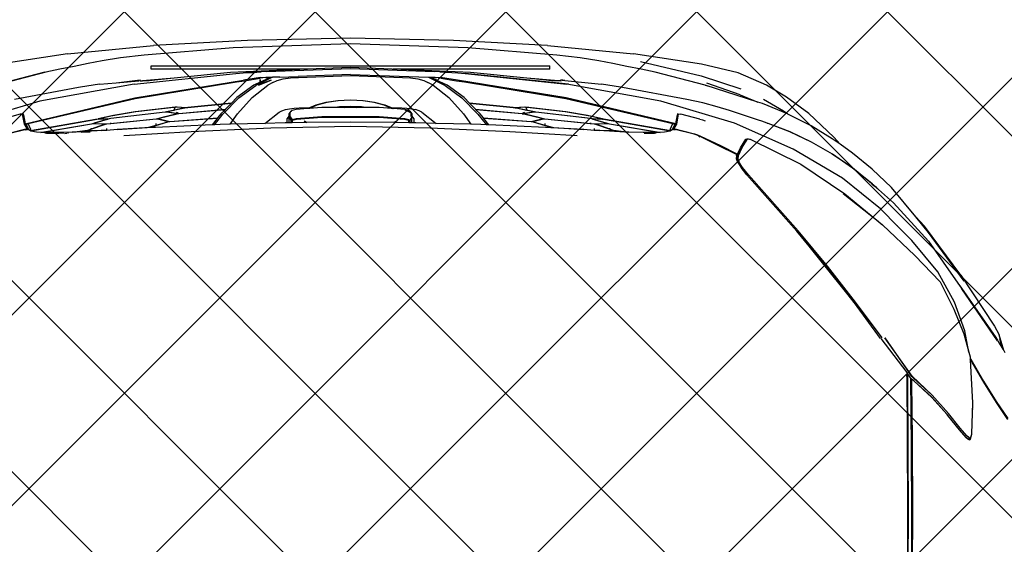
# Model space of a CAD drawing. Units: inches. Extents: x 2167 to 2589, y 1680 to 2489.
# Tile 22 of 38: x 2269 to 2306, y 1815 to 1835. Entities that reach past the tile are written whole.
import ezdxf

# ---------------------------------------------------------------- set-up
doc = ezdxf.new("R2010")
doc.units = ezdxf.units.IN
doc.header["$MEASUREMENT"] = 0
doc.layers.get('0').update_dxf_attribs({"color": 250})
for name, color, linetype, lineweight in [('A-ANNO-DIMS', 2, 'Continuous', 18), ('C-PRKG-VEHS', 8, 'Continuous', 13), ('L-PVMT-PATT', 252, 'Continuous', 13)]:
    doc.layers.add(name, color=color, linetype=linetype, lineweight=lineweight)
doc.layers.add('Edges', color=250, linetype='Continuous')
doc.styles.get("Standard").update_dxf_attribs({"font": 'arial.ttf'})
doc.dimstyles.get("Standard").update_dxf_attribs({"dimtxt": 7, "dimasz": 0.18, "dimexe": 0.18, "dimexo": 0.0625, "dimgap": 0.09, "dimtad": 0, "dimtih": 1, "dimtoh": 1, "dimdec": 1, "dimzin": 0, "dimdsep": 46, "dimlunit": 3, "dimtxsty": 'Standard', "dimcen": 0.09, "dimadec": 0, "dimazin": 0, "dimtfac": 1, "dimtdec": 1, "dimtofl": 0, "dimtmove": 0, "dimatfit": 3, "dimfxl": 1, "dimtolj": 1, "dimtzin": 0, "dimarcsym": 0})

# ---------------------------------------------------------------- blocks, each defined once
blk = doc.blocks.new('Nissan Qashqai pl')
at = {"layer": 'Edges'}
for p, q in [((7.6926, 12.7737), (7.6721, 12.7679)), ((7.6911, 12.7728), (7.6926, 12.7737)), ((7.6926, 12.7737), (7.6953, 12.7753)), ((7.7591, 12.7641), (7.7814, 12.7791)), ((7.7828, 12.7793), (7.7606, 12.7644)), ((7.5946, 12.718), (7.6608, 12.7617)), ((7.6113, 12.7186), (7.6759, 12.7633)), ((7.6799, 12.7658), (7.6125, 12.719)), ((7.6608, 12.7617), (7.6712, 12.7675)), ((7.6712, 12.7675), (7.6721, 12.7679)), ((7.6759, 12.7633), (7.6793, 12.7657)), ((7.6911, 12.7728), (7.6774, 12.7688)), ((7.6793, 12.7657), (7.6802, 12.766)), ((7.6799, 12.7658), (7.6802, 12.766)), ((7.6802, 12.766), (7.6809, 12.7664)), ((7.6809, 12.7664), (7.6911, 12.7728)), ((7.7325, 12.7476), (7.7591, 12.7641)), ((7.7606, 12.7644), (7.7341, 12.7478)), ((7.7341, 12.7478), (7.7056, 12.7314)), ((7.7038, 12.731), (7.7325, 12.7476)), ((7.6024, 12.7221), (7.5387, 12.6759)), ((7.667, 12.723), (7.6295, 12.7097)), ((7.6949, 12.7283), (7.667, 12.723)), ((7.6708, 12.7217), (7.6949, 12.7283)), ((7.6949, 12.7283), (7.701, 12.73)), ((7.701, 12.73), (7.7024, 12.7301)), ((7.7024, 12.7301), (7.7038, 12.731)), ((7.7024, 12.7301), (7.7034, 12.7301)), ((7.7056, 12.7314), (7.7034, 12.7301)), ((7.7034, 12.7301), (7.7048, 12.7302)), ((7.7048, 12.7302), (7.7608, 12.7329)), ((7.7058, 12.7308), (7.7048, 12.7302)), ((7.7608, 12.7329), (7.8014, 12.7318)), ((7.7688, 12.7328), (7.7688, 12.734)), ((7.8045, 12.7263), (7.7938, 12.7171)), ((7.8062, 12.725), (7.7959, 12.7161)), ((7.8014, 12.7318), (7.8022, 12.7316)), ((7.8022, 12.7316), (7.8037, 12.7315)), ((7.8022, 12.7316), (7.8072, 12.73)), ((7.8037, 12.7315), (7.8096, 12.7294)), ((7.8072, 12.73), (7.8045, 12.7263)), ((7.8062, 12.725), (7.8087, 12.7283)), ((7.8066, 12.7254), (7.8062, 12.725)), ((7.8096, 12.7294), (7.8066, 12.7254)), ((7.8072, 12.73), (7.8087, 12.7283)), ((7.5946, 12.718), (7.5304, 12.6704)), ((7.5501, 12.6757), (7.6051, 12.7139)), ((7.6295, 12.7097), (7.59, 12.6877)), ((7.6051, 12.7139), (7.6113, 12.7186)), ((7.6051, 12.7139), (7.6111, 12.7181)), ((7.6118, 12.7186), (7.6111, 12.7181)), ((7.6125, 12.719), (7.6118, 12.7186)), ((7.6386, 12.7089), (7.6708, 12.7217)), ((7.7938, 12.7171), (7.7748, 12.7018)), ((7.7959, 12.7161), (7.7772, 12.7011)), ((7.6032, 12.6908), (7.6386, 12.7089)), ((7.7748, 12.7018), (7.7507, 12.6803)), ((7.753, 12.6794), (7.776, 12.6999)), ((7.776, 12.6999), (7.7539, 12.68)), ((7.7772, 12.7011), (7.776, 12.6999)), ((7.59, 12.6877), (7.5492, 12.654)), ((7.5687, 12.6579), (7.6032, 12.6908)), ((7.5501, 12.6757), (7.5001, 12.6302)), ((7.5387, 12.6759), (7.5184, 12.6591)), ((7.7261, 12.6543), (7.7507, 12.6803)), ((7.753, 12.6794), (7.7281, 12.6524)), ((7.7507, 12.6803), (7.7286, 12.6561)), ((7.7539, 12.68), (7.7324, 12.6565)), ((7.5184, 12.6591), (7.4801, 12.6274)), ((7.5184, 12.6591), (7.5304, 12.6704)), ((7.5289, 12.6158), (7.5687, 12.6579)), ((7.5492, 12.654), (7.531, 12.6359)), ((7.7261, 12.6543), (7.6762, 12.6186)), ((7.6762, 12.6186), (7.7233, 12.6514)), ((7.6771, 12.6135), (7.7215, 12.6473)), ((7.7215, 12.6473), (7.7221, 12.6478)), ((7.7232, 12.6486), (7.7221, 12.6478)), ((7.7281, 12.6524), (7.7232, 12.6486)), ((7.7245, 12.6486), (7.7232, 12.6486)), ((7.7267, 12.6539), (7.7233, 12.6514)), ((7.7261, 12.6476), (7.7238, 12.6476)), ((7.7294, 12.6487), (7.7245, 12.6486)), ((7.7279, 12.6477), (7.7261, 12.6476)), ((7.7286, 12.6561), (7.7267, 12.6539)), ((7.8048, 12.6483), (7.7279, 12.6477)), ((7.7299, 12.6537), (7.7281, 12.6524)), ((7.7281, 12.6524), (7.7349, 12.6524)), ((7.731, 12.6487), (7.7294, 12.6487)), ((7.7324, 12.6565), (7.7299, 12.6537)), ((7.7299, 12.6537), (7.7334, 12.6537)), ((7.764, 12.6489), (7.731, 12.6487)), ((7.7334, 12.6537), (7.8083, 12.6544)), ((7.7349, 12.6524), (7.768, 12.6527)), ((7.7662, 12.6489), (7.764, 12.6489)), ((7.7811, 12.649), (7.7662, 12.6489)), ((7.768, 12.6527), (7.7692, 12.6527)), ((7.7692, 12.6527), (7.7844, 12.6528)), ((7.7822, 12.649), (7.7811, 12.649)), ((7.8057, 12.6491), (7.7822, 12.649)), ((7.7844, 12.6528), (7.8078, 12.653)), ((7.9014, 12.6487), (7.8048, 12.6483)), ((7.8233, 12.6492), (7.8057, 12.6491)), ((7.8078, 12.653), (7.8233, 12.6531)), ((7.8083, 12.6544), (7.904, 12.6547)), ((7.8233, 12.6531), (7.9036, 12.6534)), ((7.902, 12.6495), (7.8233, 12.6492)), ((8.0273, 12.6485), (7.9014, 12.6487)), ((8.0275, 12.6493), (7.902, 12.6495)), ((7.9036, 12.6534), (8.0275, 12.6533)), ((7.904, 12.6547), (8.0276, 12.6545)), ((7.531, 12.6359), (7.5081, 12.6131)), ((7.531, 12.6359), (7.5301, 12.6353)), ((7.4801, 12.6274), (7.4565, 12.6023)), ((7.4827, 12.6103), (7.5001, 12.6302)), ((7.5081, 12.6131), (7.4679, 12.5634)), ((7.4744, 12.6015), (7.4804, 12.6079)), ((7.4804, 12.6079), (7.478, 12.6049)), ((7.479, 12.6061), (7.4815, 12.6089)), ((7.479, 12.6061), (7.4801, 12.6074)), ((7.4801, 12.6074), (7.4804, 12.6079)), ((7.4804, 12.6079), (7.4807, 12.6082)), ((7.4804, 12.6079), (7.4804, 12.6079)), ((7.4807, 12.6082), (7.4821, 12.6097)), ((7.4815, 12.6089), (7.4821, 12.6097)), ((7.4821, 12.6097), (7.4827, 12.6103)), ((7.4882, 12.5645), (7.5243, 12.6101)), ((7.4884, 12.5664), (7.5289, 12.6158)), ((7.5243, 12.6101), (7.5286, 12.6146)), ((7.676, 12.6152), (7.6296, 12.5803)), ((7.6769, 12.6129), (7.6306, 12.5791)), ((7.4565, 12.6023), (7.4354, 12.5766)), ((7.4542, 12.5765), (7.4744, 12.6015)), ((7.475, 12.6016), (7.4549, 12.5767)), ((7.4762, 12.6028), (7.475, 12.6016)), ((7.4752, 12.6016), (7.4762, 12.6028)), ((7.4762, 12.6028), (7.478, 12.6049)), ((7.478, 12.6049), (7.479, 12.6061)), ((7.4354, 12.5766), (7.4239, 12.5604)), ((7.4363, 12.5502), (7.4542, 12.5765)), ((7.4549, 12.5767), (7.4369, 12.5504)), ((7.6296, 12.5803), (7.5827, 12.5441)), ((7.618, 12.5691), (7.5829, 12.5411)), ((7.618, 12.5691), (7.584, 12.5429)), ((7.6301, 12.5787), (7.618, 12.5691)), ((7.6306, 12.5791), (7.6301, 12.5787)), ((7.4239, 12.5604), (7.4147, 12.5524)), ((7.4239, 12.5604), (7.4166, 12.5503)), ((7.4679, 12.5634), (7.4302, 12.4993)), ((7.4498, 12.5093), (7.4884, 12.5664)), ((7.4147, 12.5524), (7.3837, 12.5197)), ((7.4166, 12.5503), (7.3997, 12.5227)), ((7.4205, 12.5229), (7.4363, 12.5502)), ((7.4369, 12.5504), (7.4211, 12.5232)), ((7.5827, 12.5441), (7.5369, 12.5057)), ((7.584, 12.5429), (7.5568, 12.5201)), ((7.5829, 12.5411), (7.5568, 12.5201)), ((7.3837, 12.5197), (7.3624, 12.4907)), ((7.3997, 12.5227), (7.3845, 12.4925)), ((7.4071, 12.4948), (7.4205, 12.5229)), ((7.4211, 12.5232), (7.4078, 12.4951)), ((7.5568, 12.5201), (7.5371, 12.5042)), ((7.4172, 12.4431), (7.4498, 12.5093)), ((7.5369, 12.5057), (7.4635, 12.4408)), ((7.4638, 12.439), (7.5371, 12.5042)), ((7.3843, 12.492), (7.3707, 12.4592)), ((7.3843, 12.492), (7.3805, 12.4866)), ((7.3845, 12.4925), (7.3843, 12.492)), ((7.3962, 12.466), (7.4071, 12.4948)), ((7.4302, 12.4993), (7.3963, 12.4227)), ((7.4078, 12.4951), (7.3969, 12.4665)), ((7.3624, 12.4907), (7.347, 12.4644)), ((7.3805, 12.4866), (7.3655, 12.4604)), ((7.3965, 12.4655), (7.3951, 12.462)), ((7.3965, 12.4655), (7.3962, 12.466)), ((7.3969, 12.4665), (7.3965, 12.4655)), ((7.347, 12.4644), (7.3309, 12.4276)), ((7.3688, 12.4532), (7.3467, 12.3846)), ((7.3596, 12.4302), (7.3688, 12.4532)), ((7.3707, 12.4592), (7.3688, 12.4532)), ((7.3925, 12.4542), (7.3845, 12.4306)), ((7.3938, 12.4583), (7.3925, 12.4542)), ((7.3951, 12.462), (7.3938, 12.4583)), ((7.3968, 12.4649), (7.3967, 12.4651)), ((7.4167, 12.4393), (7.4169, 12.4406)), ((7.4169, 12.4412), (7.4172, 12.4431)), ((7.4169, 12.4406), (7.4172, 12.4423)), ((7.4169, 12.4406), (7.4169, 12.4412)), ((7.4169, 12.4398), (7.4169, 12.4406)), ((7.4282, 12.4328), (7.4169, 12.4398)), ((7.4172, 12.4395), (7.4169, 12.4398)), ((7.4172, 12.4423), (7.4174, 12.4429)), ((7.4175, 12.4429), (7.4174, 12.4429)), ((7.4635, 12.4408), (7.4541, 12.4333)), ((7.3309, 12.4276), (7.3193, 12.3797)), ((7.3345, 12.3793), (7.3514, 12.4308)), ((7.3596, 12.4302), (7.344, 12.3869)), ((7.3845, 12.4306), (7.3799, 12.4164)), ((7.4167, 12.4393), (7.4172, 12.4395)), ((7.417, 12.4377), (7.4167, 12.4393)), ((7.4283, 12.4307), (7.417, 12.4377)), ((7.4183, 12.4382), (7.4172, 12.4395)), ((7.4183, 12.4382), (7.4296, 12.4312)), ((7.4255, 12.4044), (7.4367, 12.4268)), ((7.4387, 12.428), (7.4282, 12.4328)), ((7.4359, 12.4272), (7.4283, 12.4307)), ((7.4383, 12.4272), (7.4296, 12.4312)), ((7.4367, 12.4268), (7.4359, 12.4272)), ((7.4367, 12.4268), (7.4383, 12.4272)), ((7.4379, 12.4263), (7.4383, 12.4272)), ((7.4379, 12.4263), (7.4389, 12.4269)), ((7.4383, 12.4272), (7.4389, 12.4269)), ((7.4389, 12.4269), (7.4384, 12.426)), ((7.4431, 12.4276), (7.4387, 12.428)), ((7.44, 12.4264), (7.4389, 12.4269)), ((7.4477, 12.427), (7.443, 12.4254)), ((7.4479, 12.4293), (7.4431, 12.4276)), ((7.4442, 12.4258), (7.4477, 12.427)), ((7.4477, 12.427), (7.4541, 12.4313)), ((7.4541, 12.4333), (7.4479, 12.4293)), ((7.4638, 12.439), (7.4541, 12.4313)), ((7.3963, 12.4227), (7.3676, 12.3269)), ((7.3799, 12.4164), (7.375, 12.4)), ((7.4365, 12.4235), (7.4267, 12.4041)), ((7.4378, 12.4261), (7.4365, 12.4235)), ((7.4365, 12.4235), (7.4365, 12.4235)), ((7.4379, 12.4263), (7.4378, 12.4261)), ((7.4384, 12.426), (7.4379, 12.4263)), ((7.4384, 12.426), (7.438, 12.4251)), ((7.4387, 12.4259), (7.4384, 12.426)), ((7.443, 12.4254), (7.4387, 12.4259)), ((7.44, 12.4264), (7.4442, 12.4258)), ((7.4131, 12.3783), (7.4255, 12.4044)), ((7.4267, 12.4041), (7.4139, 12.3778)), ((7.3467, 12.3846), (7.3489, 12.3925)), ((7.375, 12.4), (7.3699, 12.3813)), ((7.3193, 12.3797), (7.3059, 12.291)), ((7.3161, 12.3001), (7.3345, 12.3793)), ((7.3467, 12.3846), (7.33, 12.3192)), ((7.3699, 12.3813), (7.3653, 12.3604)), ((7.3913, 12.3774), (7.3844, 12.3526)), ((7.3913, 12.3774), (7.3914, 12.3775)), ((7.3925, 12.3813), (7.3914, 12.3775)), ((7.3937, 12.3851), (7.3925, 12.3813)), ((7.4115, 12.3746), (7.4131, 12.3783)), ((7.4139, 12.3778), (7.4122, 12.3742)), ((7.4133, 12.3759), (7.4142, 12.3776)), ((7.4033, 12.3435), (7.4101, 12.3708)), ((7.4108, 12.3703), (7.4042, 12.3435)), ((7.4101, 12.3708), (7.4115, 12.3746)), ((7.4122, 12.3742), (7.4108, 12.3703)), ((7.3653, 12.3604), (7.3497, 12.2767)), ((7.3841, 12.3485), (7.3844, 12.3526)), ((7.3971, 12.3461), (7.3635, 12.2033)), ((7.364, 12.2029), (7.3968, 12.3424)), ((7.3846, 12.3495), (7.3841, 12.3485)), ((7.3841, 12.3485), (7.3853, 12.3483)), ((7.3846, 12.3495), (7.3976, 12.347)), ((7.3971, 12.3461), (7.3853, 12.3483)), ((7.3916, 12.2547), (7.4062, 12.3389)), ((7.4065, 12.3392), (7.3917, 12.2547)), ((7.3968, 12.3424), (7.398, 12.3449)), ((7.4046, 12.3389), (7.3968, 12.3424)), ((7.3983, 12.3458), (7.3971, 12.3461)), ((7.3976, 12.347), (7.4026, 12.3439)), ((7.398, 12.3449), (7.3999, 12.344)), ((7.398, 12.3449), (7.4012, 12.3441)), ((7.4012, 12.3441), (7.3983, 12.3458)), ((7.3999, 12.344), (7.4051, 12.3415)), ((7.3999, 12.344), (7.4048, 12.3417)), ((7.4033, 12.3427), (7.4012, 12.3441)), ((7.4012, 12.3441), (7.4015, 12.344)), ((7.4015, 12.344), (7.4028, 12.3437)), ((7.4026, 12.3439), (7.4033, 12.3435)), ((7.4033, 12.3435), (7.4042, 12.3422)), ((7.4042, 12.3422), (7.4033, 12.3427)), ((7.4042, 12.3435), (7.404, 12.3429)), ((7.404, 12.3429), (7.4043, 12.3428)), ((7.404, 12.3429), (7.4043, 12.3425)), ((7.4041, 12.3435), (7.4042, 12.3435)), ((7.4042, 12.3435), (7.4045, 12.3434)), ((7.4042, 12.3422), (7.4043, 12.3425)), ((7.4044, 12.3422), (7.4042, 12.3422)), ((7.4043, 12.3428), (7.4045, 12.3434)), ((7.4043, 12.3428), (7.4046, 12.3425)), ((7.4043, 12.3425), (7.4043, 12.3428)), ((7.4043, 12.3425), (7.4044, 12.3422)), ((7.4044, 12.3422), (7.4046, 12.3419)), ((7.4046, 12.3422), (7.4044, 12.3422)), ((7.4045, 12.3434), (7.405, 12.3456)), ((7.4045, 12.3434), (7.4048, 12.3433)), ((7.4046, 12.3425), (7.4047, 12.3424)), ((7.4047, 12.3424), (7.4046, 12.3422)), ((7.4046, 12.3422), (7.4046, 12.3419)), ((7.4048, 12.3422), (7.4046, 12.3422)), ((7.4046, 12.3419), (7.405, 12.3419)), ((7.4048, 12.3417), (7.4046, 12.3419)), ((7.4046, 12.3389), (7.4062, 12.3389)), ((7.4047, 12.3424), (7.4048, 12.3422)), ((7.4048, 12.3422), (7.405, 12.3419)), ((7.4048, 12.3417), (7.4052, 12.3416)), ((7.4051, 12.3415), (7.4048, 12.3417)), ((7.405, 12.3419), (7.4052, 12.3416)), ((7.4051, 12.3415), (7.4052, 12.3415)), ((7.4052, 12.3416), (7.4052, 12.3415)), ((7.4052, 12.3415), (7.4063, 12.3395)), ((7.4062, 12.3389), (7.4063, 12.3395)), ((7.4063, 12.3395), (7.4065, 12.3392)), ((7.4065, 12.3392), (7.4066, 12.3389)), ((7.4066, 12.3389), (7.408, 12.3313)), ((7.3676, 12.3269), (7.3455, 12.2042)), ((7.3971, 12.2599), (7.4083, 12.3258)), ((7.4084, 12.3244), (7.3975, 12.2599)), ((7.408, 12.3313), (7.4083, 12.3258)), ((7.4083, 12.3258), (7.4084, 12.3244)), ((7.4084, 12.3244), (7.4087, 12.3195)), ((7.33, 12.3192), (7.3261, 12.3009)), ((7.4087, 12.3195), (7.4087, 12.3037)), ((7.4092, 12.3184), (7.4091, 12.3206)), ((7.4092, 12.305), (7.4092, 12.3184)), ((7.3261, 12.3009), (7.3223, 12.2825)), ((7.4087, 12.3037), (7.4081, 12.2848)), ((7.2951, 12.1791), (7.3059, 12.291)), ((7.3223, 12.2825), (7.3186, 12.2641)), ((7.3494, 12.2741), (7.3457, 12.2495)), ((7.3498, 12.2768), (7.3494, 12.2741)), ((7.3497, 12.2767), (7.3494, 12.2741)), ((7.4054, 12.2651), (7.4081, 12.2848)), ((7.4079, 12.2798), (7.4059, 12.2651)), ((7.4079, 12.2798), (7.4069, 12.2598)), ((7.4081, 12.2838), (7.4079, 12.2798)), ((7.4081, 12.2848), (7.4081, 12.2838)), ((7.3186, 12.2641), (7.3149, 12.2457)), ((7.3967, 12.2579), (7.3971, 12.2599)), ((7.3975, 12.2599), (7.3973, 12.258)), ((7.4048, 12.2612), (7.3982, 12.2419)), ((7.3983, 12.244), (7.4038, 12.2599)), ((7.4028, 12.2599), (7.4038, 12.2599)), ((7.4038, 12.2599), (7.4049, 12.2631)), ((7.4053, 12.2622), (7.4048, 12.2612)), ((7.4049, 12.2631), (7.4054, 12.2651)), ((7.4053, 12.2612), (7.4053, 12.2622)), ((7.4061, 12.2473), (7.4053, 12.2612)), ((7.4059, 12.2618), (7.4056, 12.2621)), ((7.4059, 12.2651), (7.4058, 12.2632)), ((7.4058, 12.2632), (7.4059, 12.2618)), ((7.4059, 12.2618), (7.4064, 12.2523)), ((7.3407, 12.2016), (7.3457, 12.2495)), ((7.3909, 12.2508), (7.3864, 12.231)), ((7.3869, 12.2347), (7.3912, 12.2527)), ((7.3901, 12.2368), (7.391, 12.2507)), ((7.3914, 12.2527), (7.3906, 12.2386)), ((7.3908, 12.2366), (7.3965, 12.256)), ((7.3911, 12.2518), (7.3909, 12.2508)), ((7.391, 12.2387), (7.3967, 12.2579)), ((7.391, 12.2507), (7.3911, 12.2518)), ((7.3912, 12.2517), (7.3911, 12.2518)), ((7.3912, 12.2527), (7.3916, 12.2547)), ((7.3917, 12.2547), (7.3914, 12.2527)), ((7.3969, 12.257), (7.3965, 12.256)), ((7.3968, 12.2559), (7.3969, 12.257)), ((7.3972, 12.2421), (7.3968, 12.2559)), ((7.3973, 12.258), (7.3977, 12.2439)), ((7.4061, 12.2472), (7.4057, 12.24)), ((7.4064, 12.2523), (7.4061, 12.2473)), ((7.4061, 12.2472), (7.4061, 12.2473)), ((7.4069, 12.2598), (7.4064, 12.2523)), ((7.3149, 12.2457), (7.3113, 12.2217)), ((7.3813, 12.2021), (7.3869, 12.2347)), ((7.3815, 12.1638), (7.3899, 12.2348)), ((7.3903, 12.2347), (7.382, 12.1639)), ((7.3899, 12.2348), (7.3901, 12.2368)), ((7.3908, 12.2366), (7.3903, 12.2347)), ((7.3905, 12.1754), (7.3966, 12.2347)), ((7.3906, 12.2386), (7.3907, 12.2376)), ((7.3907, 12.2376), (7.391, 12.2387)), ((7.3977, 12.24), (7.3911, 12.1755)), ((7.3957, 12.2348), (7.3966, 12.2348)), ((7.3957, 12.2347), (7.3966, 12.2347)), ((7.3966, 12.2348), (7.3972, 12.24)), ((7.3966, 12.2347), (7.3966, 12.2348)), ((7.3972, 12.24), (7.3972, 12.2421)), ((7.3977, 12.2439), (7.398, 12.2429)), ((7.3982, 12.2419), (7.3977, 12.24)), ((7.398, 12.2429), (7.3983, 12.244)), ((7.4032, 12.24), (7.4057, 12.24)), ((7.4057, 12.24), (7.4048, 12.2262)), ((7.3113, 12.2217), (7.3078, 12.191)), ((7.3864, 12.231), (7.3815, 12.2029)), ((7.4022, 12.187), (7.4048, 12.2262)), ((7.4048, 12.2262), (7.4023, 12.1836)), ((7.4072, 12.1299), (7.4124, 12.2176)), ((7.3455, 12.2062), (7.3317, 12.0717)), ((7.3317, 12.0717), (7.3455, 12.2042)), ((7.3407, 12.2016), (7.34, 12.1962)), ((7.34, 12.1962), (7.3401, 12.1962)), ((7.3401, 12.1962), (7.341, 12.1962)), ((7.3403, 12.1981), (7.3407, 12.2016)), ((7.3635, 12.2033), (7.3405, 12.0616)), ((7.341, 12.1962), (7.3414, 12.1962)), ((7.341, 12.1962), (7.341, 12.1962)), ((7.3414, 12.1962), (7.341, 12.1962)), ((7.341, 12.1962), (7.3413, 12.1933)), ((7.3426, 12.0707), (7.364, 12.2029)), ((7.375, 12.1484), (7.3813, 12.2021)), ((7.3815, 12.2029), (7.3756, 12.1509)), ((7.3078, 12.191), (7.298, 12.075)), ((7.3407, 12.1879), (7.3378, 12.1521)), ((7.341, 12.1848), (7.34, 12.1731)), ((7.3413, 12.1933), (7.3407, 12.1879)), ((7.3413, 12.1931), (7.341, 12.1848)), ((7.3415, 12.1954), (7.3413, 12.1933)), ((7.3413, 12.1933), (7.3413, 12.1931)), ((7.4021, 12.1833), (7.3951, 12.1606)), ((7.399, 12.1756), (7.4017, 12.185)), ((7.4017, 12.185), (7.4022, 12.187)), ((7.4023, 12.1836), (7.4018, 12.1764)), ((7.4023, 12.1836), (7.4021, 12.1833)), ((7.2951, 12.1791), (7.2884, 12.0562)), ((7.3261, 12.1821), (7.3216, 12.1821)), ((7.3216, 11.6621), (7.3216, 12.1821)), ((7.3261, 12.1821), (7.3261, 11.9779)), ((7.34, 12.1731), (7.3378, 12.1521)), ((7.3903, 12.1716), (7.3844, 12.1479)), ((7.3877, 12.1639), (7.3901, 12.1734)), ((7.3901, 12.1734), (7.3905, 12.1754)), ((7.3907, 12.1727), (7.3903, 12.1716)), ((7.3909, 12.1716), (7.3907, 12.1727)), ((7.3939, 12.1596), (7.3909, 12.1716)), ((7.3911, 12.1755), (7.3913, 12.1737)), ((7.3913, 12.1737), (7.3943, 12.1614)), ((7.3949, 12.1616), (7.399, 12.1756)), ((7.3967, 12.1756), (7.399, 12.1756)), ((7.4018, 12.1764), (7.3986, 12.1025)), ((7.3813, 12.1599), (7.3763, 12.1361)), ((7.3792, 12.1518), (7.3812, 12.1619)), ((7.3812, 12.1619), (7.3815, 12.1638)), ((7.3815, 12.161), (7.3813, 12.1599)), ((7.3817, 12.16), (7.3815, 12.161)), ((7.3832, 12.1493), (7.3817, 12.16)), ((7.382, 12.1639), (7.382, 12.1619)), ((7.382, 12.1619), (7.3838, 12.1497)), ((7.3843, 12.1498), (7.3877, 12.1639)), ((7.3877, 12.1639), (7.3874, 12.1639)), ((7.3896, 12.0954), (7.3941, 12.1576)), ((7.3945, 12.1577), (7.3903, 12.0959)), ((7.3941, 12.1576), (7.3939, 12.1596)), ((7.3943, 12.1614), (7.3947, 12.1605)), ((7.3951, 12.1606), (7.3945, 12.1577)), ((7.3947, 12.1605), (7.3949, 12.1616)), ((7.3378, 12.1521), (7.3302, 12.0785)), ((7.376, 12.136), (7.375, 12.1484)), ((7.3756, 12.1509), (7.3792, 12.1518)), ((7.3756, 12.1509), (7.3762, 12.138)), ((7.3764, 12.138), (7.3792, 12.1518)), ((7.3783, 12.0852), (7.3836, 12.1459)), ((7.384, 12.1459), (7.3788, 12.0857)), ((7.3832, 12.1493), (7.3824, 12.1487)), ((7.3824, 12.1487), (7.3832, 12.1492)), ((7.3836, 12.1459), (7.3824, 12.1487)), ((7.3824, 12.1487), (7.3835, 12.1468)), ((7.3838, 12.1497), (7.3832, 12.1493)), ((7.3832, 12.1492), (7.3837, 12.1495)), ((7.3832, 12.1492), (7.3832, 12.1493)), ((7.3836, 12.1459), (7.3835, 12.1468)), ((7.3835, 12.1468), (7.384, 12.1459)), ((7.3837, 12.1495), (7.3843, 12.1498)), ((7.3837, 12.1495), (7.3838, 12.1497)), ((7.384, 12.1459), (7.3842, 12.1495)), ((7.3844, 12.1479), (7.384, 12.1459)), ((7.3842, 12.1495), (7.3843, 12.1498)), ((7.3843, 12.1495), (7.3842, 12.1495)), ((7.3701, 12.0771), (7.3759, 12.1341)), ((7.3761, 12.1341), (7.3704, 12.0773)), ((7.3759, 12.1341), (7.376, 12.136)), ((7.3763, 12.1361), (7.3761, 12.1341)), ((7.3762, 12.137), (7.3764, 12.138)), ((7.3762, 12.138), (7.3762, 12.137)), ((7.3764, 12.1371), (7.3762, 12.137)), ((7.4025, 12.026), (7.4072, 12.1299)), ((7.3896, 12.0954), (7.3841, 12.091)), ((7.3845, 12.0883), (7.3985, 12.0993)), ((7.3903, 12.0959), (7.3896, 12.0954)), ((7.3986, 12.1025), (7.3903, 12.0959)), ((7.3985, 12.0993), (7.3982, 12.092)), ((7.3986, 12.1025), (7.3985, 12.0993)), ((7.3633, 12.0674), (7.3845, 12.0883)), ((7.3783, 12.0852), (7.3704, 12.0773)), ((7.3788, 12.0857), (7.3783, 12.0852)), ((7.3841, 12.091), (7.3788, 12.0857)), ((7.3982, 12.092), (7.3978, 12.0791)), ((7.298, 12.075), (7.2928, 11.9221)), ((7.3302, 12.0785), (7.3261, 11.9779)), ((7.3309, 12.0619), (7.3317, 12.0717)), ((7.341, 12.0605), (7.3426, 12.0707)), ((7.3631, 12.0701), (7.3469, 12.0481)), ((7.3471, 12.0454), (7.3633, 12.0674)), ((7.363, 12.0501), (7.3842, 12.0693)), ((7.3701, 12.0771), (7.3631, 12.0701)), ((7.3704, 12.0773), (7.3701, 12.0771)), ((7.3842, 12.0693), (7.3978, 12.0791)), ((7.3978, 12.0791), (7.3966, 12.0338)), ((7.2884, 12.0562), (7.2857, 11.9221)), ((7.3294, 12.0385), (7.3309, 12.0619)), ((7.3405, 12.0616), (7.3369, 12.0394)), ((7.3377, 12.0398), (7.341, 12.0605)), ((7.3365, 12.0237), (7.3471, 12.0454)), ((7.3469, 12.0481), (7.3402, 12.0337)), ((7.3468, 12.0299), (7.363, 12.0501)), ((7.3251, 11.9221), (7.3291, 12.0316)), ((7.3294, 12.0385), (7.3291, 12.0316)), ((7.3362, 12.0248), (7.3365, 12.0321)), ((7.3365, 12.0321), (7.3369, 12.0394)), ((7.3377, 12.0398), (7.3369, 12.0328)), ((7.3369, 12.0287), (7.3369, 12.0328)), ((7.338, 12.0291), (7.3369, 12.0287)), ((7.338, 12.0291), (7.3374, 12.0276)), ((7.3402, 12.0337), (7.338, 12.0291)), ((7.3387, 12.0332), (7.3402, 12.0337)), ((7.3468, 12.0299), (7.3432, 12.0231)), ((7.3818, 12.0151), (7.3966, 12.0338)), ((7.3966, 12.0338), (7.3959, 12.0071)), ((7.3329, 11.9221), (7.3365, 12.0237)), ((7.3362, 12.0248), (7.3366, 12.0246)), ((7.3365, 12.0237), (7.3362, 12.0248)), ((7.3374, 12.0276), (7.3369, 12.0287)), ((7.3386, 12.01), (7.3407, 12.0176)), ((7.3407, 12.0176), (7.3432, 12.0231)), ((7.4002, 11.9221), (7.4025, 12.026)), ((7.3373, 12.0004), (7.3386, 12.01)), ((7.3775, 12.0015), (7.3786, 12.007)), ((7.3801, 12.0115), (7.3786, 12.007)), ((7.3818, 12.0151), (7.3801, 12.0115)), ((7.3909, 12.0051), (7.387, 12.0021)), ((7.3956, 12.0051), (7.3909, 12.0051)), ((7.3959, 12.0049), (7.3956, 12.0051)), ((7.3959, 12.0051), (7.3956, 12.0051)), ((7.3959, 12.0049), (7.3958, 12.0018)), ((7.3959, 12.0071), (7.3959, 12.0051)), ((7.3959, 12.0051), (7.3959, 12.0049)), ((7.3367, 11.99), (7.3373, 12.0004)), ((7.3765, 11.989), (7.3768, 11.9954)), ((7.3768, 11.9954), (7.3775, 12.0015)), ((7.3787, 11.9928), (7.3774, 11.9778)), ((7.3798, 11.9983), (7.3787, 11.9928)), ((7.3787, 11.9928), (7.38, 11.9953)), ((7.3808, 11.9993), (7.3798, 11.9983)), ((7.3807, 11.9991), (7.3798, 11.9983)), ((7.38, 11.9953), (7.383, 12.0011)), ((7.3807, 11.9991), (7.3808, 11.9993)), ((7.381, 11.9993), (7.3807, 11.9991)), ((7.3808, 11.9993), (7.384, 12.0021)), ((7.381, 11.9993), (7.3808, 11.9993)), ((7.383, 12.0011), (7.381, 11.9993)), ((7.3866, 12.0011), (7.383, 12.0011)), ((7.384, 12.0021), (7.387, 12.0021)), ((7.3868, 12.002), (7.3866, 12.0011)), ((7.3875, 12.0011), (7.3866, 12.0011)), ((7.387, 12.0021), (7.3868, 12.002)), ((7.387, 12.0021), (7.3885, 12.0021)), ((7.3876, 11.9595), (7.3904, 11.9928)), ((7.3885, 12.0021), (7.3925, 11.9993)), ((7.3955, 12.0021), (7.3885, 12.0021)), ((7.3917, 11.9926), (7.3889, 11.9594)), ((7.3904, 11.9928), (7.3916, 11.9983)), ((7.3929, 11.9981), (7.3917, 11.9926)), ((7.3925, 11.9993), (7.3958, 11.9993)), ((7.3925, 11.9993), (7.3929, 11.9981)), ((7.3958, 11.9981), (7.3929, 11.9981)), ((7.3955, 12.0021), (7.3958, 12.0018)), ((7.3958, 11.9981), (7.3956, 11.9801)), ((7.3958, 12.0018), (7.3958, 11.9993)), ((7.3958, 11.9993), (7.3958, 11.9981)), ((7.3261, 11.9764), (7.3261, 11.9779)), ((7.3343, 11.9221), (7.3367, 11.99)), ((7.3761, 11.9751), (7.3765, 11.989)), ((7.3774, 11.9778), (7.3771, 11.9771)), ((7.3774, 11.9774), (7.3774, 11.9778)), ((7.3938, 11.9823), (7.3956, 11.9801)), ((7.3956, 11.9788), (7.3938, 11.981)), ((7.3956, 11.9788), (7.3951, 11.9221)), ((7.3956, 11.9801), (7.3956, 11.9788)), ((7.3261, 11.9764), (7.3238, 11.9221)), ((7.369, 11.9536), (7.3724, 11.9667)), ((7.3727, 11.9658), (7.3693, 11.953)), ((7.3724, 11.9667), (7.3761, 11.9751)), ((7.3771, 11.9757), (7.3727, 11.9658)), ((7.3773, 11.9759), (7.3759, 11.9595)), ((7.3761, 11.9751), (7.3769, 11.9767)), ((7.3769, 11.9767), (7.3771, 11.977)), ((7.3771, 11.9771), (7.3774, 11.9774)), ((7.3771, 11.9771), (7.3771, 11.977)), ((7.3773, 11.9759), (7.3771, 11.9757)), ((7.3774, 11.9774), (7.3773, 11.9759)), ((7.3668, 11.9384), (7.369, 11.9536)), ((7.3693, 11.953), (7.3672, 11.9381)), ((7.3759, 11.9595), (7.3759, 11.9417)), ((7.3876, 11.8847), (7.3876, 11.9595)), ((7.3889, 11.9594), (7.3889, 11.8848)), ((7.3759, 11.9417), (7.3751, 11.9363)), ((7.3759, 11.9417), (7.3759, 11.9303)), ((7.3661, 11.9221), (7.3668, 11.9384)), ((7.3672, 11.9381), (7.3665, 11.9221)), ((7.3751, 11.9363), (7.3745, 11.9221)), ((7.3755, 11.9221), (7.3759, 11.9303)), ((7.3759, 11.9303), (7.3759, 11.9139)), ((7.2857, 11.9221), (7.2884, 11.7879)), ((7.2928, 11.9221), (7.298, 11.7692)), ((7.3238, 11.9221), (7.3261, 11.8662)), ((7.3291, 11.8126), (7.3251, 11.9221)), ((7.3329, 11.9221), (7.3354, 11.8539)), ((7.3367, 11.8541), (7.3343, 11.9221)), ((7.3668, 11.9057), (7.3661, 11.9221)), ((7.3665, 11.9221), (7.3672, 11.9061)), ((7.3745, 11.9221), (7.3751, 11.9078)), ((7.3759, 11.9139), (7.3755, 11.9221)), ((7.3759, 11.9139), (7.3759, 11.9025)), ((7.3951, 11.9221), (7.3956, 11.8653)), ((7.4025, 11.8181), (7.4002, 11.9221)), ((7.369, 11.8905), (7.3668, 11.9057)), ((7.3672, 11.9061), (7.3693, 11.8911)), ((7.3751, 11.9078), (7.3759, 11.9025)), ((7.3759, 11.9025), (7.3759, 11.8847)), ((7.3724, 11.8775), (7.369, 11.8905)), ((7.3693, 11.8911), (7.3727, 11.8783)), ((7.3761, 11.8691), (7.3724, 11.8775)), ((7.3727, 11.8783), (7.3771, 11.8685)), ((7.3759, 11.8847), (7.3773, 11.8682)), ((7.3904, 11.8513), (7.3876, 11.8847)), ((7.3889, 11.8848), (7.3917, 11.8516)), ((7.3261, 11.8662), (7.3302, 11.7656)), ((7.3261, 11.8662), (7.3261, 11.6621)), ((7.3765, 11.8551), (7.3761, 11.8691)), ((7.3769, 11.8674), (7.3761, 11.8691)), ((7.3771, 11.8671), (7.3769, 11.8674)), ((7.3771, 11.8685), (7.3773, 11.8682)), ((7.3771, 11.8671), (7.3771, 11.8671)), ((7.3771, 11.8671), (7.3774, 11.8664)), ((7.3774, 11.8668), (7.3771, 11.8671)), ((7.3773, 11.8682), (7.3774, 11.8668)), ((7.3774, 11.8668), (7.3774, 11.8664)), ((7.3774, 11.8664), (7.3787, 11.8513)), ((7.3938, 11.8632), (7.3956, 11.8653)), ((7.3956, 11.864), (7.3938, 11.8619)), ((7.3956, 11.8653), (7.3956, 11.864)), ((7.3956, 11.864), (7.3958, 11.8461)), ((7.3361, 11.8416), (7.3354, 11.8539)), ((7.3373, 11.8438), (7.3367, 11.8541)), ((7.3768, 11.8488), (7.3765, 11.8551)), ((7.3787, 11.8513), (7.3798, 11.8459)), ((7.3916, 11.8459), (7.3904, 11.8513)), ((7.3917, 11.8516), (7.3929, 11.8461)), ((7.3362, 11.8301), (7.3361, 11.8416)), ((7.3386, 11.8342), (7.3373, 11.8438)), ((7.3775, 11.8427), (7.3768, 11.8488)), ((7.3786, 11.8372), (7.3775, 11.8427)), ((7.3801, 11.8327), (7.3786, 11.8372)), ((7.3798, 11.8459), (7.3808, 11.8448)), ((7.3808, 11.8448), (7.3807, 11.8451)), ((7.3808, 11.8448), (7.381, 11.8448)), ((7.384, 11.8421), (7.3808, 11.8448)), ((7.383, 11.8431), (7.3875, 11.8431)), ((7.387, 11.8421), (7.384, 11.8421)), ((7.387, 11.8421), (7.3909, 11.8391)), ((7.3885, 11.8421), (7.387, 11.8421)), ((7.3875, 11.8431), (7.3916, 11.8459)), ((7.3925, 11.8448), (7.3885, 11.8421)), ((7.3955, 11.8421), (7.3885, 11.8421)), ((7.3909, 11.8391), (7.3956, 11.8391)), ((7.3929, 11.8461), (7.3925, 11.8448)), ((7.3958, 11.8448), (7.3925, 11.8448)), ((7.3929, 11.8461), (7.3958, 11.8461)), ((7.3958, 11.8423), (7.3955, 11.8421)), ((7.3956, 11.8391), (7.3959, 11.8392)), ((7.3956, 11.8391), (7.3959, 11.8391)), ((7.3958, 11.8461), (7.3958, 11.8448)), ((7.3958, 11.8448), (7.3958, 11.8423)), ((7.3958, 11.8423), (7.3959, 11.8392)), ((7.3959, 11.8392), (7.3959, 11.8391)), ((7.3959, 11.8391), (7.3959, 11.8371)), ((7.3959, 11.8371), (7.3966, 11.8103)), ((7.3362, 11.8301), (7.3365, 11.8204)), ((7.3407, 11.8266), (7.3386, 11.8342)), ((7.3432, 11.821), (7.3407, 11.8266)), ((7.3818, 11.8291), (7.3801, 11.8327)), ((7.3966, 11.8103), (7.3818, 11.8291)), ((7.3291, 11.8126), (7.3294, 11.8057)), ((7.3362, 11.8194), (7.3365, 11.8204)), ((7.3367, 11.8196), (7.3362, 11.8194)), ((7.3365, 11.812), (7.3362, 11.8194)), ((7.3365, 11.8204), (7.3471, 11.7987)), ((7.3369, 11.8047), (7.3365, 11.812)), ((7.3369, 11.8155), (7.3374, 11.8165)), ((7.3369, 11.8113), (7.3369, 11.8155)), ((7.3369, 11.8155), (7.338, 11.8151)), ((7.3369, 11.8113), (7.3377, 11.8044)), ((7.3374, 11.8165), (7.338, 11.8151)), ((7.338, 11.8151), (7.343, 11.8045)), ((7.3401, 11.8186), (7.3431, 11.8112)), ((7.347, 11.8021), (7.3401, 11.8186)), ((7.3431, 11.8112), (7.347, 11.8021)), ((7.3432, 11.821), (7.3468, 11.8142)), ((7.363, 11.794), (7.3468, 11.8142)), ((7.4072, 11.7142), (7.4025, 11.8181)), ((7.3301, 11.7949), (7.3294, 11.8057)), ((7.3295, 11.8012), (7.3309, 11.7822)), ((7.3295, 11.8012), (7.3301, 11.7949)), ((7.3369, 11.8047), (7.3405, 11.7825)), ((7.3377, 11.8042), (7.3377, 11.8044)), ((7.341, 11.7837), (7.3377, 11.8042)), ((7.343, 11.8045), (7.3396, 11.8043)), ((7.3396, 11.8043), (7.3431, 11.8042)), ((7.343, 11.8045), (7.3431, 11.8042)), ((7.3431, 11.8042), (7.3469, 11.7961)), ((7.3633, 11.7767), (7.3471, 11.7987)), ((7.3966, 11.8103), (7.3978, 11.7651)), ((7.2884, 11.7879), (7.2951, 11.6651)), ((7.3309, 11.7822), (7.3301, 11.7949)), ((7.3469, 11.7961), (7.3631, 11.774)), ((7.3842, 11.7749), (7.363, 11.794)), ((7.3317, 11.7724), (7.3309, 11.7822)), ((7.3455, 11.64), (7.3317, 11.7724)), ((7.3635, 11.6409), (7.3405, 11.7825)), ((7.3426, 11.7735), (7.341, 11.7837)), ((7.364, 11.6413), (7.3426, 11.7735)), ((7.3631, 11.774), (7.3701, 11.7671)), ((7.3845, 11.7558), (7.3633, 11.7767)), ((7.3978, 11.7651), (7.3842, 11.7749)), ((7.298, 11.7692), (7.3078, 11.6532)), ((7.3302, 11.7656), (7.3378, 11.6921)), ((7.3759, 11.7101), (7.3701, 11.7671)), ((7.3701, 11.7671), (7.3704, 11.7668)), ((7.3704, 11.7668), (7.3761, 11.71)), ((7.3704, 11.7668), (7.3783, 11.759)), ((7.3978, 11.7651), (7.3982, 11.7521)), ((7.3836, 11.6983), (7.3783, 11.759)), ((7.3783, 11.759), (7.3788, 11.7585)), ((7.3788, 11.7585), (7.384, 11.6982)), ((7.3788, 11.7585), (7.3841, 11.7532)), ((7.3841, 11.7532), (7.3896, 11.7488)), ((7.3985, 11.7448), (7.3845, 11.7558)), ((7.3941, 11.6865), (7.3896, 11.7488)), ((7.3896, 11.7488), (7.3903, 11.7483)), ((7.3903, 11.7483), (7.3945, 11.6865)), ((7.3903, 11.7483), (7.3986, 11.7417)), ((7.3982, 11.7521), (7.3985, 11.7448)), ((7.3985, 11.7448), (7.3986, 11.7417)), ((7.3986, 11.7417), (7.4018, 11.6678)), ((7.375, 11.6957), (7.376, 11.7081)), ((7.376, 11.7081), (7.3759, 11.7101)), ((7.3761, 11.71), (7.3763, 11.7081)), ((7.3763, 11.7081), (7.3813, 11.6842)), ((7.4124, 11.6265), (7.4072, 11.7142)), ((7.3813, 11.642), (7.375, 11.6957)), ((7.3757, 11.6959), (7.3756, 11.6933)), ((7.3762, 11.7062), (7.3757, 11.6959)), ((7.3757, 11.6959), (7.3757, 11.6959)), ((7.3762, 11.7062), (7.3764, 11.7061)), ((7.3764, 11.7061), (7.3792, 11.6924)), ((7.3824, 11.6955), (7.3836, 11.6983)), ((7.3835, 11.6973), (7.3824, 11.6955)), ((7.3834, 11.6959), (7.3824, 11.6955)), ((7.3824, 11.6955), (7.3832, 11.6949)), ((7.3832, 11.695), (7.3824, 11.6955)), ((7.3832, 11.695), (7.3834, 11.6959)), ((7.3838, 11.6947), (7.3832, 11.695)), ((7.3837, 11.696), (7.3834, 11.6959)), ((7.3835, 11.6973), (7.3836, 11.6983)), ((7.3836, 11.6975), (7.3835, 11.6973)), ((7.3836, 11.6975), (7.3836, 11.6983)), ((7.384, 11.6982), (7.3836, 11.6975)), ((7.3844, 11.6963), (7.3837, 11.696)), ((7.3838, 11.6947), (7.3837, 11.696)), ((7.3843, 11.6944), (7.3844, 11.6963)), ((7.3844, 11.6963), (7.3903, 11.6725)), ((7.3378, 11.6921), (7.3407, 11.6563)), ((7.3378, 11.6921), (7.34, 11.671)), ((7.3792, 11.6924), (7.3756, 11.6933)), ((7.3756, 11.6933), (7.3815, 11.6413)), ((7.3812, 11.6823), (7.3792, 11.6924)), ((7.3815, 11.6804), (7.3812, 11.6823)), ((7.3813, 11.6842), (7.3817, 11.6844)), ((7.3817, 11.6841), (7.3813, 11.6842)), ((7.3817, 11.6844), (7.3832, 11.6949)), ((7.3817, 11.6841), (7.3817, 11.6844)), ((7.3838, 11.6944), (7.382, 11.6823)), ((7.382, 11.6823), (7.382, 11.6803)), ((7.3832, 11.6949), (7.3838, 11.6944)), ((7.3843, 11.6944), (7.3838, 11.6947)), ((7.3843, 11.6942), (7.3838, 11.6944)), ((7.3843, 11.6942), (7.3843, 11.6944)), ((7.3877, 11.6803), (7.3843, 11.6942)), ((7.3909, 11.6728), (7.3939, 11.6846)), ((7.3943, 11.6827), (7.3913, 11.6705)), ((7.3939, 11.6846), (7.3941, 11.6865)), ((7.3943, 11.6827), (7.3949, 11.6826)), ((7.3943, 11.6827), (7.395, 11.6825)), ((7.3945, 11.6865), (7.3951, 11.6835)), ((7.395, 11.6825), (7.3949, 11.6826)), ((7.399, 11.6686), (7.395, 11.6825)), ((7.3951, 11.6835), (7.4021, 11.6609)), ((7.34, 11.671), (7.341, 11.6594)), ((7.3899, 11.6094), (7.3815, 11.6804)), ((7.382, 11.6803), (7.3903, 11.6095)), ((7.3874, 11.6803), (7.3877, 11.6803)), ((7.3901, 11.6707), (7.3877, 11.6803)), ((7.3905, 11.6687), (7.3901, 11.6707)), ((7.3909, 11.6728), (7.3903, 11.6725)), ((7.3909, 11.6725), (7.3903, 11.6725)), ((7.3909, 11.6725), (7.3909, 11.6728)), ((7.3913, 11.6705), (7.3911, 11.6687)), ((7.3059, 11.5532), (7.2951, 11.6651)), ((7.3261, 11.6621), (7.3216, 11.6621)), ((7.341, 11.6594), (7.3413, 11.6511)), ((7.3966, 11.6095), (7.3905, 11.6687)), ((7.3911, 11.6687), (7.3977, 11.6042)), ((7.399, 11.6686), (7.3967, 11.6686)), ((7.4017, 11.6592), (7.399, 11.6686)), ((7.4022, 11.6571), (7.4017, 11.6592)), ((7.4018, 11.6678), (7.4022, 11.6609)), ((7.4022, 11.6609), (7.4021, 11.6609)), ((7.4022, 11.6609), (7.4021, 11.6609)), ((7.4022, 11.6609), (7.4048, 11.618)), ((7.4022, 11.6609), (7.4022, 11.6609)), ((7.4048, 11.618), (7.4022, 11.6571)), ((7.3078, 11.6532), (7.3113, 11.6224)), ((7.3401, 11.648), (7.34, 11.648)), ((7.3438, 11.6167), (7.34, 11.648)), ((7.341, 11.648), (7.3401, 11.648)), ((7.3407, 11.6563), (7.3413, 11.6509)), ((7.341, 11.648), (7.3413, 11.6509)), ((7.3414, 11.648), (7.341, 11.648)), ((7.341, 11.648), (7.3414, 11.648)), ((7.3438, 11.6167), (7.3412, 11.646)), ((7.3413, 11.6511), (7.3413, 11.6509)), ((7.3413, 11.6509), (7.3415, 11.6488)), ((7.3455, 11.64), (7.3676, 11.5172)), ((7.3971, 11.4981), (7.3635, 11.6409)), ((7.3968, 11.5018), (7.364, 11.6413)), ((7.3869, 11.6094), (7.3813, 11.642)), ((7.3815, 11.6413), (7.3864, 11.6131)), ((7.3113, 11.6224), (7.3149, 11.5984)), ((7.4048, 11.618), (7.4057, 11.6042)), ((7.3457, 11.5947), (7.3438, 11.6167)), ((7.3864, 11.6131), (7.3909, 11.5933)), ((7.3912, 11.5914), (7.3869, 11.6094)), ((7.3901, 11.6073), (7.3899, 11.6094)), ((7.391, 11.5935), (7.3901, 11.6073)), ((7.3903, 11.6095), (7.3908, 11.6076)), ((7.3906, 11.6055), (7.391, 11.6055)), ((7.3906, 11.6055), (7.391, 11.6054)), ((7.3906, 11.6055), (7.3914, 11.5914)), ((7.3908, 11.6076), (7.3965, 11.5881)), ((7.391, 11.6054), (7.391, 11.6055)), ((7.3967, 11.5862), (7.391, 11.6054)), ((7.3966, 11.6095), (7.3957, 11.6095)), ((7.3972, 11.6042), (7.3966, 11.6095)), ((7.3149, 11.5984), (7.3186, 11.58)), ((7.3457, 11.5947), (7.3494, 11.57)), ((7.391, 11.5935), (7.3909, 11.5933)), ((7.391, 11.5934), (7.3909, 11.5933)), ((7.3968, 11.5882), (7.3972, 11.6021)), ((7.3972, 11.6021), (7.3972, 11.6042)), ((7.3977, 11.6003), (7.3973, 11.5862)), ((7.3977, 11.6042), (7.3982, 11.6022)), ((7.3977, 11.6003), (7.3983, 11.6002)), ((7.3977, 11.6003), (7.3983, 11.6001)), ((7.3982, 11.6022), (7.4048, 11.5829)), ((7.3983, 11.6001), (7.3983, 11.6002)), ((7.4038, 11.5843), (7.3983, 11.6001)), ((7.4057, 11.6042), (7.4032, 11.6042)), ((7.4053, 11.5831), (7.4061, 11.5969)), ((7.4057, 11.6042), (7.4061, 11.597)), ((7.4061, 11.5969), (7.4061, 11.597)), ((7.4061, 11.5969), (7.4064, 11.5919)), ((7.3186, 11.58), (7.3223, 11.5616)), ((7.3916, 11.5894), (7.3912, 11.5914)), ((7.3914, 11.5914), (7.3917, 11.5895)), ((7.4062, 11.5053), (7.3916, 11.5894)), ((7.3917, 11.5895), (7.4065, 11.505)), ((7.3968, 11.5882), (7.3965, 11.5881)), ((7.3971, 11.5842), (7.3967, 11.5862)), ((7.3968, 11.5882), (7.3973, 11.5884)), ((7.4083, 11.5184), (7.3971, 11.5842)), ((7.3973, 11.5862), (7.3975, 11.5843)), ((7.3975, 11.5843), (7.4084, 11.5198)), ((7.4038, 11.5843), (7.4028, 11.5843)), ((7.4049, 11.5811), (7.4038, 11.5843)), ((7.4053, 11.5831), (7.4048, 11.5829)), ((7.4053, 11.583), (7.4048, 11.5829)), ((7.4054, 11.5791), (7.4049, 11.5811)), ((7.406, 11.5834), (7.4053, 11.5831)), ((7.406, 11.5833), (7.4053, 11.583)), ((7.4053, 11.583), (7.4053, 11.5831)), ((7.406, 11.5833), (7.4058, 11.581)), ((7.4058, 11.581), (7.4059, 11.579)), ((7.4064, 11.5919), (7.406, 11.5834)), ((7.406, 11.5834), (7.406, 11.5833)), ((7.4064, 11.5919), (7.4069, 11.5844)), ((7.4069, 11.5844), (7.4079, 11.5644)), ((7.4081, 11.5711), (7.4075, 11.5828)), ((7.3494, 11.57), (7.3497, 11.5674)), ((7.3494, 11.57), (7.3498, 11.5674)), ((7.3497, 11.5674), (7.3653, 11.4838)), ((7.4081, 11.5593), (7.4054, 11.5791)), ((7.4059, 11.579), (7.4079, 11.5644)), ((7.3223, 11.5616), (7.3261, 11.5433)), ((7.4079, 11.5644), (7.4081, 11.5604)), ((7.4079, 11.5644), (7.4081, 11.5629)), ((7.4081, 11.5604), (7.4081, 11.5593)), ((7.4081, 11.5593), (7.4087, 11.5405)), ((7.4093, 11.5546), (7.4095, 11.5529)), ((7.3059, 11.5532), (7.3193, 11.4645)), ((7.3261, 11.5433), (7.33, 11.5249)), ((7.4092, 11.5416), (7.409, 11.5485)), ((7.4096, 11.549), (7.4092, 11.5521)), ((7.4092, 11.5258), (7.4092, 11.5416)), ((7.4087, 11.5405), (7.4087, 11.5246)), ((7.3297, 11.5237), (7.3467, 11.4596)), ((7.33, 11.5249), (7.3467, 11.4596)), ((7.3676, 11.5172), (7.3963, 11.4215)), ((7.4083, 11.5184), (7.408, 11.5129)), ((7.4084, 11.5198), (7.4083, 11.5184)), ((7.4087, 11.5246), (7.4084, 11.5198)), ((7.4091, 11.5235), (7.4092, 11.5258)), ((7.4046, 11.5053), (7.3968, 11.5018)), ((7.398, 11.4993), (7.4048, 11.5024)), ((7.4062, 11.5053), (7.4046, 11.5053)), ((7.4046, 11.5023), (7.4048, 11.5024)), ((7.4048, 11.5024), (7.4052, 11.5027)), ((7.4052, 11.5026), (7.4048, 11.5024)), ((7.4052, 11.5026), (7.405, 11.5023)), ((7.4063, 11.5047), (7.4052, 11.5027)), ((7.4052, 11.5027), (7.4052, 11.5026)), ((7.4063, 11.5047), (7.4062, 11.5053)), ((7.4065, 11.505), (7.4063, 11.5047)), ((7.4066, 11.5052), (7.4065, 11.505)), ((7.408, 11.5129), (7.4066, 11.5052)), ((7.3853, 11.4958), (7.3841, 11.4956)), ((7.3844, 11.4916), (7.3841, 11.4956)), ((7.3846, 11.4946), (7.3844, 11.4916)), ((7.3844, 11.4916), (7.3914, 11.4667)), ((7.3976, 11.4971), (7.3846, 11.4946)), ((7.3853, 11.4958), (7.3846, 11.4946)), ((7.3853, 11.4958), (7.3971, 11.4981)), ((7.398, 11.4993), (7.3968, 11.5018)), ((7.3971, 11.4981), (7.3983, 11.4983)), ((7.4026, 11.5002), (7.3976, 11.4971)), ((7.4012, 11.5001), (7.398, 11.4993)), ((7.3983, 11.4983), (7.4012, 11.5001)), ((7.4012, 11.5001), (7.4033, 11.5014)), ((7.403, 11.5005), (7.4026, 11.5002)), ((7.403, 11.5005), (7.4028, 11.5004)), ((7.4033, 11.5007), (7.403, 11.5005)), ((7.4033, 11.5014), (7.4042, 11.502)), ((7.4042, 11.502), (7.4033, 11.5007)), ((7.4033, 11.5005), (7.4033, 11.5007)), ((7.4034, 11.5005), (7.4033, 11.5005)), ((7.4101, 11.4733), (7.4033, 11.5005)), ((7.4043, 11.5016), (7.404, 11.5012)), ((7.4043, 11.5014), (7.404, 11.5012)), ((7.404, 11.5012), (7.4108, 11.4738)), ((7.4042, 11.502), (7.4044, 11.502)), ((7.4043, 11.5016), (7.4042, 11.502)), ((7.4044, 11.502), (7.4043, 11.5016)), ((7.4046, 11.5016), (7.4043, 11.5014)), ((7.4043, 11.5014), (7.4043, 11.5016)), ((7.4045, 11.5008), (7.4043, 11.5014)), ((7.4046, 11.5023), (7.4044, 11.502)), ((7.4044, 11.502), (7.4046, 11.502)), ((7.4048, 11.5008), (7.4045, 11.5008)), ((7.405, 11.4985), (7.4045, 11.5008)), ((7.405, 11.5023), (7.4046, 11.5023)), ((7.4046, 11.5023), (7.4046, 11.502)), ((7.4046, 11.502), (7.4047, 11.5018)), ((7.4046, 11.502), (7.4048, 11.502)), ((7.4047, 11.5018), (7.4046, 11.5016)), ((7.4048, 11.502), (7.4047, 11.5018)), ((7.405, 11.5023), (7.4048, 11.502))]:
    blk.add_line(p, q, dxfattribs=at)
blk = doc.blocks.new('car')
blk.add_blockref('Nissan Qashqai pl', (-9.7433, -11.9151))
blk = doc.blocks.new('carr')
blk.add_blockref('car', (0.5124, -0.007))
blk = doc.blocks.new('*D45')
at = {"layer": 'A-ANNO-DIMS', "color": 0, "lineweight": -2, "transparency": 16777216}
for p, q in [((2251.156, 1833.955), (2232.359, 1833.955)), ((2232.539, 1833.775), (2232.539, 1775.399)), ((2232.539, 1709.605), (2232.539, 1767.981)), ((2251.156, 1709.425), (2232.359, 1709.425))]:
    blk.add_line(p, q, dxfattribs=at)
at = {"layer": 'A-ANNO-DIMS', "color": 0, "transparency": 16777216}
for points in [[(2232.509, 1833.775), (2232.569, 1833.775), (2232.539, 1833.955)], [(2232.509, 1709.605), (2232.569, 1709.605), (2232.539, 1709.425)]]:
    blk.add_solid(points, dxfattribs=at)
at = {"layer": 'Defpoints', "color": 0, "transparency": 16777216}
for p in [(2251.218, 1833.955), (2232.539, 1709.425), (2251.218, 1709.425)]:
    blk.add_point(p, dxfattribs=at)
at = {"layer": 'A-ANNO-DIMS', "color": 0, "transparency": 16777216, "insert": (2232.539, 1771.69), "char_height": 7, "attachment_point": 5}
blk.add_mtext('\\A1;CAR 10\'-4 1/2" TYP.', dxfattribs=at)

msp = doc.modelspace()

# ---------------------------------------------------------------- hatches: boundary and pattern name
at = {"layer": 'L-PVMT-PATT'}
h = msp.add_hatch(dxfattribs=at)
h.set_pattern_fill('ANSI37', color=256, scale=40)
h.paths.add_polyline_path([(2417.548, 1783.695), (2417.548, 1846.042), (2239.361, 1846.042), (2239.361, 1687.695), (2369.843, 1687.695), (2369.843, 1696.695), (2375.607, 1696.695), (2416.107, 1696.695), (2417.548, 1696.695)])

# ---------------------------------------------------------------- block references
at = {"layer": 'C-PRKG-VEHS', "xscale": 28.42784210623918, "yscale": 28.42784210623918, "zscale": 28.42784210623918, "rotation": 270}
msp.add_blockref('carr', (2281.736, 1778.659), dxfattribs=at)

# ---------------------------------------------------------------- dimensions: what is measured, and where the dimension line sits
at = {"layer": 'A-ANNO-DIMS'}
dim = msp.add_linear_dim(base=(2232.539, 1709.425), p1=(2251.218, 1833.955), p2=(2251.218, 1709.425), angle=270, text='CAR <> TYP.', dimstyle='Standard', override={"dimdec": 1, "dimlfac": 1, "dimrnd": 0, "dimzin": 1, "dimdsep": 46, "dimlunit": 4, "dimfrac": 2}, dxfattribs=at)
dim.commit()
dim.dimension.update_dxf_attribs({"geometry": '*D45', "text_midpoint": (2232.539, 1771.69)})

doc.saveas('drawing.dxf')
